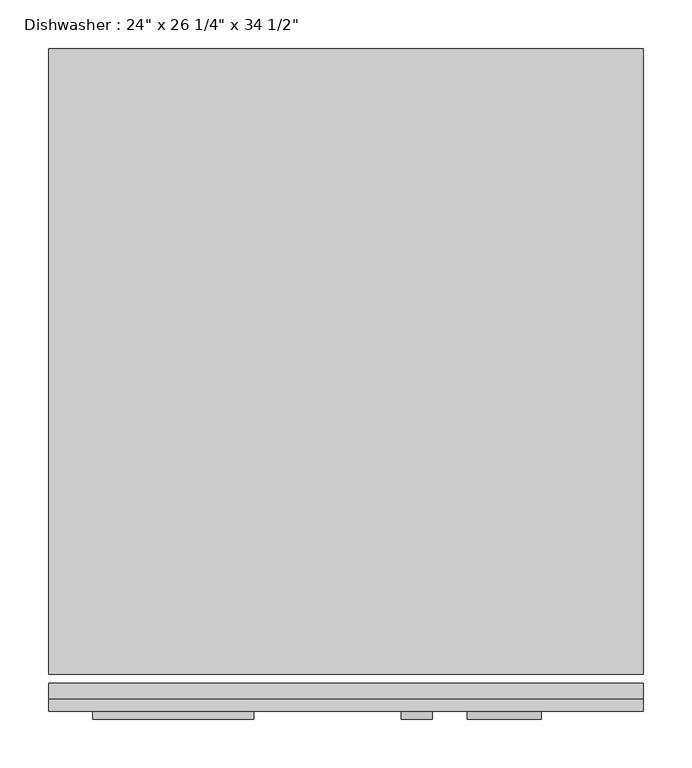
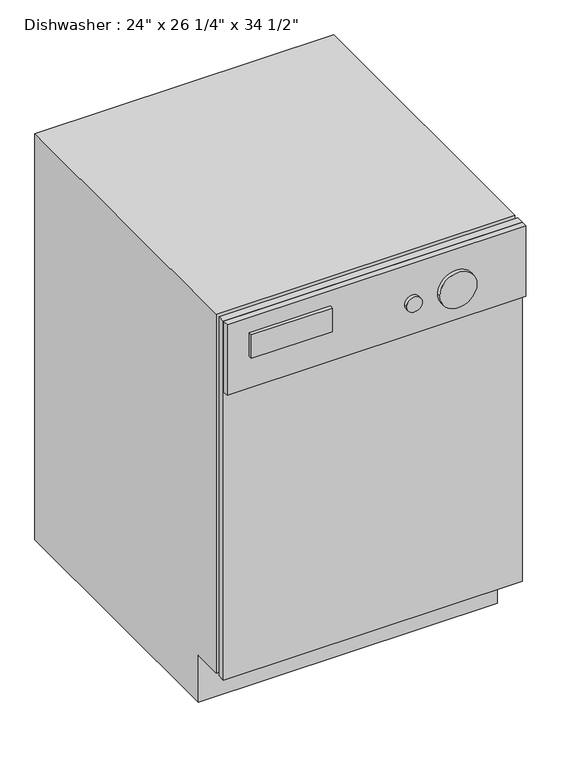
"""IFC4 building model written with IfcOpenShell, lengths in millimetres: proxy geometry."""

from ifc_helpers import new_model, si_unit, point, frame, frame_2d, origin, place, context, project, spatial, polyline, circle_curve, trimmed, segment, composite_curve, outline, extrude, source, transform, mapped, element, save


def proxy_19aded4c(model_context):
    return source(origin(), model_context, "Body", "SweptSolid", [
        extrude(outline(polyline([(687.1174685, -38.3504352), (77.5174685, -38.3504352), (77.5174685, -22.4754352), (687.1174685, -22.4754352), (687.1174685, -38.3504352)])), frame((0.0, 0.0, 101.6), z_axis=(0.0, 0.0, 1.0), x_axis=(1.0, 0.0, 0.0)), (0.0, 0.0, 1.0), 774.7),
        extrude(outline(polyline([(687.1174685, -38.3504352), (687.1174685, -51.0504352), (77.5174685, -51.0504352), (77.5174685, -38.3504352), (687.1174685, -38.3504352)])), frame((0.0, 0.0, 723.9), z_axis=(0.0, 0.0, 1.0), x_axis=(1.0, 0.0, 0.0)), (0.0, 0.0, 1.0), 152.4),
        extrude(outline(polyline([(628.3995648, 0.0), (50.5495648, 0.0), (50.5495648, 101.6), (-12.9504352, 101.6), (-12.9504352, 876.3), (628.3995648, 876.3), (628.3995648, 0.0)])), frame((77.5174685, 0.0, 0.0), z_axis=(1.0, 0.0, 0.0), x_axis=(0.0, 1.0, 0.0)), (0.0, 0.0, 1.0), 609.6),
        extrude(outline(polyline([(287.6378068, -59.1863727), (122.5378068, -59.1863727), (122.5378068, -51.0504352), (287.6378068, -51.0504352), (287.6378068, -59.1863727)])), frame((0.0, 0.0, 792.7846419), z_axis=(0.0, 0.0, 1.0), x_axis=(1.0, 0.0, 0.0)), (0.0, 0.0, 1.0), 50.8),
        extrude(outline(composite_curve([segment(trimmed(circle_curve(frame_2d((792.7846419, 544.7247133)), 38.1), [point((792.7846419, 506.6247133))], [point((792.7846419, 582.8247133))], False, "CARTESIAN"), True, "CONTINUOUS"), segment(trimmed(circle_curve(frame_2d((792.7846419, 544.7247133)), 38.1), [point((792.7846419, 582.8247133))], [point((792.7846419, 506.6247133))], False, "CARTESIAN"), True, "CONTINUOUS")], self_intersect=False)), frame((0.0, -59.1863727, 0.0), z_axis=(0.0, 1.0, 0.0), x_axis=(0.0, 0.0, 1.0)), (0.0, 0.0, 1.0), 8.1359375),
        extrude(outline(composite_curve([segment(trimmed(circle_curve(frame_2d((792.7846419, 455.195318)), 15.875), [point((792.7846419, 439.320318))], [point((792.7846419, 471.070318))], False, "CARTESIAN"), True, "CONTINUOUS"), segment(trimmed(circle_curve(frame_2d((792.7846419, 455.195318)), 15.875), [point((792.7846419, 471.070318))], [point((792.7846419, 439.320318))], False, "CARTESIAN"), True, "CONTINUOUS")], self_intersect=False)), frame((0.0, -59.1863727, 0.0), z_axis=(0.0, 1.0, 0.0), x_axis=(0.0, 0.0, 1.0)), (0.0, 0.0, 1.0), 8.1359375),
    ])


if __name__ == "__main__":
    model = new_model("IFC4")
    model_context = context("Model", 3, world=origin())
    ifc_project = project(units=[si_unit("LENGTHUNIT", "METRE", prefix="MILLI")], contexts=[model_context])
    site = spatial("IfcSite", under=ifc_project)
    building = spatial("IfcBuilding", under=site)
    placement = place(None, origin())
    proxy_shape = proxy_19aded4c(model_context)
    element("IfcBuildingElementProxy", 1, Name="Dishwasher : 24\" x 26 1/4\" x 34 1/2\"", ObjectType="Dishwasher : 24\" x 26 1/4\" x 34 1/2\"", at=placement, inside=building, context=model_context, shape_type="MappedRepresentation", body=[
        mapped(proxy_shape, transform((0.0, 0.0, 0.0), x_axis=(1.0, 0.0, 0.0), y_axis=(0.0, 1.0, 0.0), z_axis=(0.0, 0.0, 1.0))),
    ])
    save(model, "model.ifc")

# Revit data of these elements
# Type "Dishwasher : 24\" x 26 1/4\" x 34 1/2\""
#   Label = "DW"
#   Assembly Code = "E1090400"
#   Depth = 2' - 2 1/4"
#   Height = 2' - 10 1/2"
#   Width = 2' - 0"
#   Dishwasher Material = Steel, Paint Finish, Ivory, Glossy
#   Panel Face Material = Plastic, Opaque Black
#   Default Elevation = 0
# Element 1 (IfcBuildingElementProxy, "Dishwasher : 24\" x 26 1/4\" x 34 1/2\"")
#   Materials on its faces: "Steel, Paint Finish, Ivory, Glossy", "Plastic, Opaque Black"
# Materials
#   "Steel, Paint Finish, Ivory, Glossy": class "Metal", colour RGB 247 247 239, transparency 0, Description = "Steel, paint finish, ivory, glossy", Cost = 0
#   "Plastic, Opaque Black": class "Plastic", colour RGB 0 0 0, transparency 0.05, Description = "Plastic, generic, opaque black", Cost = 0
